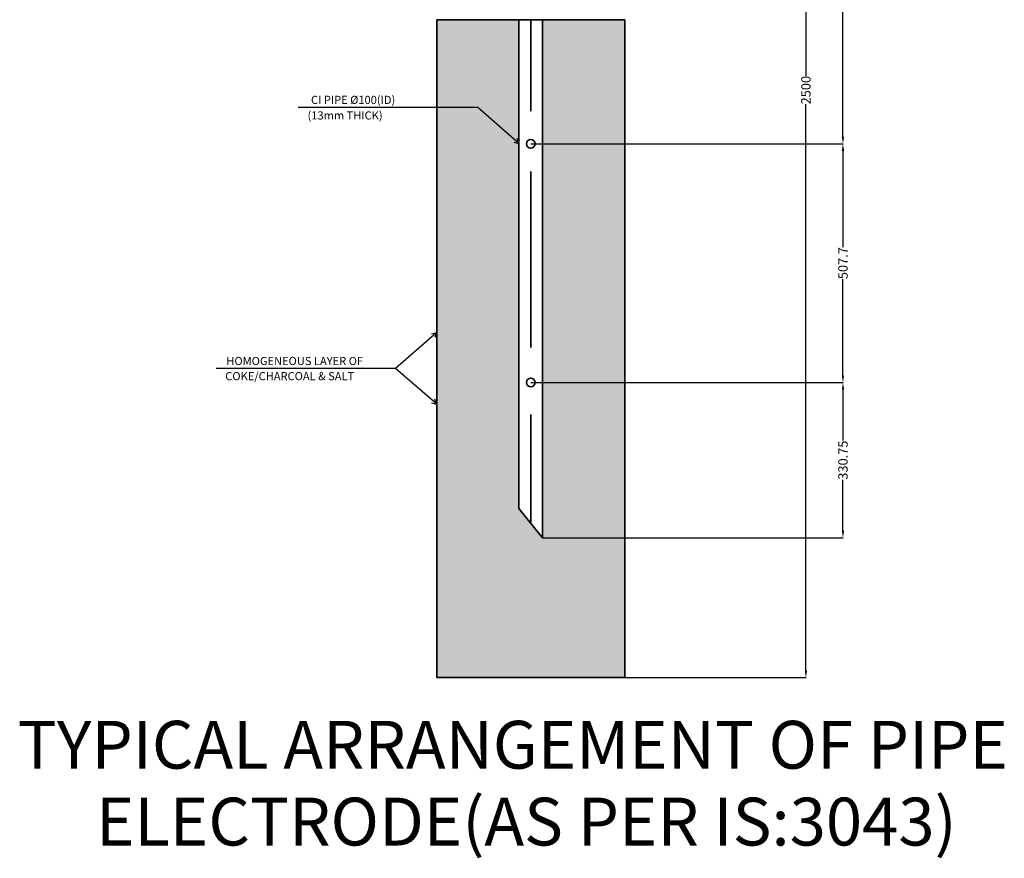
# Model space of a CAD drawing. Units: inches. Extents: x -129 to 2013, y -3652 to 814.
# Tile 1 of 5: x -82 to 2013, y -3652 to -1868. Entities that reach past the tile are written whole.
import ezdxf

# ---------------------------------------------------------------- set-up
doc = ezdxf.new("R2010")
doc.units = ezdxf.units.IN
doc.header["$MEASUREMENT"] = 0
for name, color, linetype, lineweight in [('A-ANNO-DIMS', 2, 'Continuous', 18), ('A-ANNO-TEXT', 7, 'Continuous', 25), ('A-DETL', 7, 'Continuous', 35), ('A-DETL-PATT', 8, 'Continuous', 13), ('E-GRND', 1, 'Continuous', 35)]:
    doc.layers.add(name, color=color, linetype=linetype, lineweight=lineweight)
doc.styles.get("Standard").update_dxf_attribs({"font": 'arial.ttf'})
doc.dimstyles.get("Standard").update_dxf_attribs({"dimtxt": 20, "dimasz": 15, "dimexe": 0.18, "dimexo": 0.0625, "dimgap": 0.09, "dimtad": 0, "dimdec": 0, "dimzin": 0, "dimdsep": 46, "dimtxsty": 'Standard', "dimcen": 0.09, "dimadec": 0, "dimazin": 0, "dimtfac": 1, "dimtdec": 0, "dimtofl": 0, "dimtmove": 0, "dimatfit": 3, "dimfxl": 1, "dimtolj": 1, "dimtzin": 0, "dimarcsym": 0})

# ---------------------------------------------------------------- blocks, each defined once
blk = doc.blocks.new('*D3')
at = {"layer": 'A-ANNO-DIMS', "color": 0, "lineweight": -2, "transparency": 16777216}
for p, q in [((1205.4, -767.6), (1591, -767.6)), ((1590.8, -782.6), (1590.8, -1987.5)), ((1590.8, -3252.6), (1590.8, -2047.7)), ((1205.4, -3267.6), (1591, -3267.6))]:
    blk.add_line(p, q, dxfattribs=at)
at = {"layer": 'A-ANNO-DIMS', "color": 0, "transparency": 16777216}
for points in [[(1588.3, -782.6), (1593.3, -782.6), (1590.8, -767.6)], [(1588.3, -3252.6), (1593.3, -3252.6), (1590.8, -3267.6)]]:
    blk.add_solid(points, dxfattribs=at)
at = {"layer": 'Defpoints', "color": 0, "transparency": 16777216}
for p in [(1205.3, -767.6), (1205.3, -3267.6), (1590.8, -3267.6)]:
    blk.add_point(p, dxfattribs=at)
at = {"layer": 'A-ANNO-DIMS', "color": 0, "transparency": 16777216, "insert": (1590.8, -2017.6), "char_height": 20, "attachment_point": 5, "rotation": 90}
blk.add_mtext('\\A1;2500', dxfattribs=at)
blk = doc.blocks.new('*D31')
at = {"layer": 'A-ANNO-DIMS', "color": 0, "lineweight": -2, "transparency": 16777216}
for p, q in [((1005.4, -1342.6), (1669.8, -1342.6)), ((1669.6, -1357.6), (1669.6, -1703.6)), ((1669.6, -2116.9), (1669.6, -1770.9)), ((1005.4, -2131.9), (1669.8, -2131.9))]:
    blk.add_line(p, q, dxfattribs=at)
at = {"layer": 'A-ANNO-DIMS', "color": 0, "transparency": 16777216}
for points in [[(1667.1, -1357.6), (1672.1, -1357.6), (1669.6, -1342.6)], [(1667.1, -2116.9), (1672.1, -2116.9), (1669.6, -2131.9)]]:
    blk.add_solid(points, dxfattribs=at)
at = {"layer": 'Defpoints', "color": 0, "transparency": 16777216}
for p in [(1005.3, -1342.6), (1005.3, -2131.9), (1669.6, -2131.9)]:
    blk.add_point(p, dxfattribs=at)
at = {"layer": 'A-ANNO-DIMS', "color": 0, "transparency": 16777216, "insert": (1669.6, -1737.2), "char_height": 20, "attachment_point": 5, "rotation": 90}
blk.add_mtext('\\A1;789.2', dxfattribs=at)
blk = doc.blocks.new('*D32')
at = {"layer": 'A-ANNO-DIMS', "color": 0, "lineweight": -2, "transparency": 16777216}
for p, q in [((1005.4, -2131.9), (1669.8, -2131.9)), ((1669.6, -2146.9), (1669.6, -2351.9)), ((1669.6, -2624.6), (1669.6, -2419.5)), ((1005.4, -2639.6), (1669.8, -2639.6))]:
    blk.add_line(p, q, dxfattribs=at)
at = {"layer": 'A-ANNO-DIMS', "color": 0, "transparency": 16777216}
for points in [[(1667.1, -2146.9), (1672.1, -2146.9), (1669.6, -2131.9)], [(1667.1, -2624.6), (1672.1, -2624.6), (1669.6, -2639.6)]]:
    blk.add_solid(points, dxfattribs=at)
at = {"layer": 'Defpoints', "color": 0, "transparency": 16777216}
for p in [(1005.3, -2131.9), (1005.3, -2639.6), (1669.6, -2639.6)]:
    blk.add_point(p, dxfattribs=at)
at = {"layer": 'A-ANNO-DIMS', "color": 0, "transparency": 16777216, "insert": (1669.6, -2385.7), "char_height": 20, "attachment_point": 5, "rotation": 90}
blk.add_mtext('\\A1;507.7', dxfattribs=at)
blk = doc.blocks.new('*D33')
at = {"layer": 'A-ANNO-DIMS', "color": 0, "lineweight": -2, "transparency": 16777216}
for p, q in [((1005.4, -2639.6), (1669.8, -2639.6)), ((1669.6, -2654.6), (1669.6, -2763.3)), ((1669.6, -2955.3), (1669.6, -2846.6)), ((1030.4, -2970.3), (1669.8, -2970.3))]:
    blk.add_line(p, q, dxfattribs=at)
at = {"layer": 'A-ANNO-DIMS', "color": 0, "transparency": 16777216}
for points in [[(1667.1, -2654.6), (1672.1, -2654.6), (1669.6, -2639.6)], [(1667.1, -2955.3), (1672.1, -2955.3), (1669.6, -2970.3)]]:
    blk.add_solid(points, dxfattribs=at)
at = {"layer": 'Defpoints', "color": 0, "transparency": 16777216}
for p in [(1005.3, -2639.6), (1030.3, -2970.3), (1669.6, -2970.3)]:
    blk.add_point(p, dxfattribs=at)
at = {"layer": 'A-ANNO-DIMS', "color": 0, "transparency": 16777216, "insert": (1669.6, -2804.9), "char_height": 20, "attachment_point": 5, "rotation": 90}
blk.add_mtext('\\A1;330.75', dxfattribs=at)

msp = doc.modelspace()

# ---------------------------------------------------------------- hatches: boundary and pattern name
at = {"layer": 'A-DETL-PATT'}
h = msp.add_hatch(dxfattribs=at)
h.set_pattern_fill('AR-CONC', color=256, scale=10)
h.paths.add_polyline_path([(1205.3299, -767.6397), (1030.3299, -767.6397), (1030.3299, -1767.6397), (1205.3299, -1767.6397)])
h.paths.add_polyline_path([(980.3299, -767.6397), (805.3299, -767.6397), (805.3299, -1767.6397), (980.3299, -1767.6397)])
h.paths.add_polyline_path([(980.3299, -1867.6397), (805.3299, -1867.6397), (805.3299, -3267.6397), (1205.3299, -3267.6397), (1205.3299, -1867.6397), (1030.3299, -1867.6397), (1030.3299, -2970.3227), (980.3299, -2907.6958)])

# ---------------------------------------------------------------- linework, layer by layer
at = {"layer": 'A-ANNO-TEXT'}
for p, q in [((805.3299, -2533.5458), (717.4149, -2609.6369)), ((717.4149, -2609.6369), (335.813, -2609.6369)), ((805.3299, -2685.728), (717.4149, -2609.6369))]:
    msp.add_line(p, q, dxfattribs=at)
for points in [[(980.3299, -2130.9233), (892.4149, -2054.8322), (510.813, -2054.8322)], [(969.4553, -2128.3342), (980.3299, -2130.9233), (976.215, -2120.5297)], [(794.4553, -2536.1348), (805.3299, -2533.5458), (801.215, -2543.9394)], [(794.4553, -2683.1389), (805.3299, -2685.728), (801.215, -2675.3344)]]:
    msp.add_lwpolyline(points, dxfattribs=at)
at = {"layer": 'A-DETL'}
for p, q in [((1205.3299, -1867.6397), (805.3299, -1867.6397)), ((805.3299, -1867.6397), (805.3299, -3267.6397)), ((1205.3299, -1867.6397), (1205.3299, -3267.6397)), ((1205.3299, -3267.6397), (805.3299, -3267.6397))]:
    msp.add_line(p, q, dxfattribs=at)
at = {"layer": 'E-GRND'}
for p, q in [((980.3299, -1867.6397), (980.3299, -2907.6958)), ((1005.3299, -1867.6397), (1005.3299, -2061.9631)), ((1030.3299, -1867.6397), (1030.3299, -2970.3227)), ((1005.3299, -2190.6454), (1005.3299, -2564.9059)), ((1005.3299, -2707.6724), (1005.3299, -2939.0093)), ((980.3299, -2907.6958), (1030.3299, -2970.3227))]:
    msp.add_line(p, q, dxfattribs=at)
for centre in [(1005.3299, -2131.8545), (1005.3299, -2639.57)]:
    msp.add_circle(centre, 9.277, dxfattribs=at)

# ---------------------------------------------------------------- texts
at = {"layer": 'A-ANNO-TEXT'}
for s, height, p in [('(13mm THICK)', 17.305551, (530.4261, -2080.041)), ('HOMOGENEOUS LAYER OF', 17.305551, (357.6929, -2602.5908)), ('COKE/CHARCOAL & SALT', 17.305551, (355.4261, -2634.8457)), ('TYPICAL ARRANGEMENT OF PIPE', 101.800702, (-86.2358, -3461.4843)), ('ELECTRODE(AS PER IS:3043)', 101.800702, (80.409, -3625.0182))]:
    msp.add_text(s, height=height, dxfattribs=at).set_placement(p)
at = {"layer": 'A-ANNO-TEXT', "insert": (537.8634, -2029.6204), "char_height": 17.305551, "width": 202.62979, "attachment_point": 1}
msp.add_mtext('CI PIPE %%C100(ID) ', dxfattribs=at)

# ---------------------------------------------------------------- dimensions: what is measured, and where the dimension line sits
at = {"layer": 'A-ANNO-DIMS'}
for base, p1, p2, override, picture, middle in [((1590.798, -3267.6397), (1205.3299, -767.6397), (1205.3299, -3267.6397), {"dimclrd": 0, "dimclre": 0, "dimclrt": 0}, '*D3', (1590.798, -2017.6397)), ((1669.5799, -2131.8545), (1005.3299, -1342.6284), (1005.3299, -2131.8545), {"dimdec": 1, "dimlfac": 1, "dimrnd": 0, "dimzin": 0, "dimdsep": 46, "dimlunit": 2}, '*D31', (1669.5799, -1737.2414)), ((1669.5799, -2639.57), (1005.3299, -2131.8545), (1005.3299, -2639.57), {"dimdec": 1, "dimlfac": 1, "dimrnd": 0, "dimzin": 0, "dimdsep": 46, "dimlunit": 2}, '*D32', (1669.5799, -2385.7122)), ((1669.5799, -2970.3227), (1005.3299, -2639.57), (1030.3299, -2970.3227), {"dimdec": 2, "dimlfac": 1, "dimrnd": 0, "dimzin": 0, "dimdsep": 46, "dimlunit": 2}, '*D33', (1669.5799, -2804.9464))]:
    dim = msp.add_linear_dim(base=base, p1=p1, p2=p2, angle=90, dimstyle='Standard', override=override, dxfattribs=at)
    dim.commit()
    dim.dimension.update_dxf_attribs({"geometry": picture, "text_midpoint": middle})

doc.saveas('drawing.dxf')
